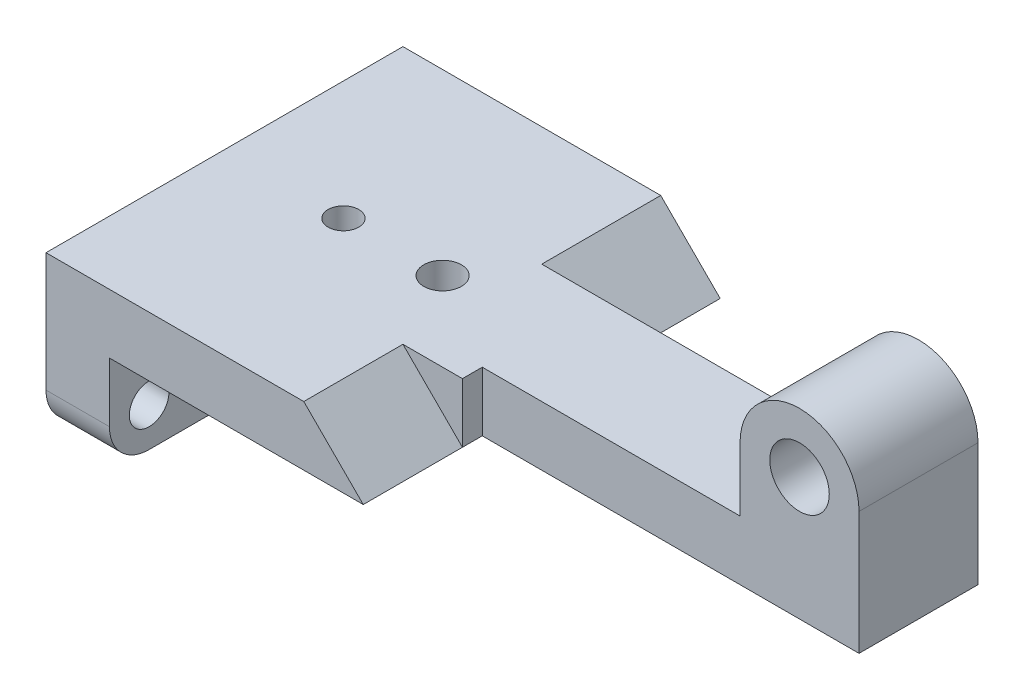
ISO-10303-21;
HEADER;
FILE_DESCRIPTION(('STEP AP214'),'2;1');
FILE_NAME('part.step','',(''),(''),'','','');
FILE_SCHEMA(('AUTOMOTIVE_DESIGN { 1 0 10303 214 1 1 1 1 }'));
ENDSEC;
DATA;
#1=APPLICATION_CONTEXT('core data for automotive mechanical design processes');
#2=APPLICATION_PROTOCOL_DEFINITION('international standard','automotive_design',2000,#1);
#3=PRODUCT_CONTEXT('',#1,'mechanical');
#4=PRODUCT('Part','Part','',(#3));
#5=PRODUCT_RELATED_PRODUCT_CATEGORY('part','',(#4));
#6=PRODUCT_DEFINITION_FORMATION('','',#4);
#7=PRODUCT_DEFINITION_CONTEXT('part definition',#1,'design');
#8=PRODUCT_DEFINITION('design','',#6,#7);
#9=PRODUCT_DEFINITION_SHAPE('','',#8);
#10=(LENGTH_UNIT() NAMED_UNIT(*) SI_UNIT(.MILLI.,.METRE.));
#11=(NAMED_UNIT(*) PLANE_ANGLE_UNIT() SI_UNIT($,.RADIAN.));
#12=(NAMED_UNIT(*) SI_UNIT($,.STERADIAN.) SOLID_ANGLE_UNIT());
#13=UNCERTAINTY_MEASURE_WITH_UNIT(LENGTH_MEASURE(1.E-05),#10,'distance_accuracy_value','');
#14=(GEOMETRIC_REPRESENTATION_CONTEXT(3) GLOBAL_UNCERTAINTY_ASSIGNED_CONTEXT((#13)) GLOBAL_UNIT_ASSIGNED_CONTEXT((#10,
#11,#12)) REPRESENTATION_CONTEXT('',''));
#15=CARTESIAN_POINT('',(0.,0.,0.));
#16=DIRECTION('',(0.,0.,1.));
#17=DIRECTION('',(1.,0.,0.));
#18=AXIS2_PLACEMENT_3D('',#15,#16,#17);
#19=CARTESIAN_POINT('',(80.,-15.,-15.));
#20=DIRECTION('',(1.,0.,0.));
#21=DIRECTION('',(0.,1.,0.));
#22=AXIS2_PLACEMENT_3D('',#19,#20,#21);
#23=PLANE('',#22);
#24=DIRECTION('',(0.,0.,-1.));
#25=VECTOR('',#24,1.);
#26=CARTESIAN_POINT('',(80.,-15.,-15.));
#27=LINE('',#26,#25);
#28=CARTESIAN_POINT('',(80.,-15.,20.));
#29=VERTEX_POINT('',#28);
#30=CARTESIAN_POINT('',(80.,-15.,15.));
#31=VERTEX_POINT('',#30);
#32=EDGE_CURVE('E206',#29,#31,#27,.T.);
#33=ORIENTED_EDGE('',*,*,#32,.T.);
#34=DIRECTION('',(0.,-1.,0.));
#35=VECTOR('',#34,1.);
#36=CARTESIAN_POINT('',(80.,-15.,15.));
#37=LINE('',#36,#35);
#38=CARTESIAN_POINT('',(80.,0.,15.));
#39=VERTEX_POINT('',#38);
#40=EDGE_CURVE('E188',#39,#31,#37,.T.);
#41=ORIENTED_EDGE('',*,*,#40,.F.);
#42=DIRECTION('',(0.,0.,-1.));
#43=VECTOR('',#42,1.);
#44=CARTESIAN_POINT('',(80.,0.,-15.));
#45=LINE('',#44,#43);
#46=CARTESIAN_POINT('',(80.,0.,20.));
#47=VERTEX_POINT('',#46);
#48=EDGE_CURVE('E214',#47,#39,#45,.T.);
#49=ORIENTED_EDGE('',*,*,#48,.F.);
#50=DIRECTION('',(0.,1.,0.));
#51=VECTOR('',#50,1.);
#52=CARTESIAN_POINT('',(80.,-15.,20.));
#53=LINE('',#52,#51);
#54=EDGE_CURVE('E208',#29,#47,#53,.T.);
#55=ORIENTED_EDGE('',*,*,#54,.F.);
#56=EDGE_LOOP('',(#33,#41,#49,#55));
#57=FACE_BOUND('',#56,.T.);
#58=ADVANCED_FACE('F39',(#57),#23,.T.);
#59=CARTESIAN_POINT('',(80.,-15.,45.));
#60=DIRECTION('',(-0.707106781186543,-0.707106781186552,0.));
#61=DIRECTION('',(0.707106781186552,-0.707106781186543,0.));
#62=AXIS2_PLACEMENT_3D('',#59,#60,#61);
#63=PLANE('',#62);
#64=DIRECTION('',(0.,0.,-1.));
#65=VECTOR('',#64,1.);
#66=CARTESIAN_POINT('',(64.9999999999998,0.,45.));
#67=LINE('',#66,#65);
#68=CARTESIAN_POINT('',(64.9999999999998,0.,-15.));
#69=VERTEX_POINT('',#68);
#70=CARTESIAN_POINT('',(64.9999999999998,0.,-45.));
#71=VERTEX_POINT('',#70);
#72=EDGE_CURVE('E233',#69,#71,#67,.T.);
#73=ORIENTED_EDGE('',*,*,#72,.F.);
#74=DIRECTION('',(0.707106781186552,-0.707106781186543,0.));
#75=VECTOR('',#74,1.);
#76=CARTESIAN_POINT('',(80.,-15.,-15.));
#77=LINE('',#76,#75);
#78=CARTESIAN_POINT('',(80.,-15.,-15.));
#79=VERTEX_POINT('',#78);
#80=EDGE_CURVE('E262',#69,#79,#77,.T.);
#81=ORIENTED_EDGE('',*,*,#80,.T.);
#82=DIRECTION('',(0.,0.,-1.));
#83=VECTOR('',#82,1.);
#84=CARTESIAN_POINT('',(80.,-15.,45.));
#85=LINE('',#84,#83);
#86=CARTESIAN_POINT('',(80.,-15.,-45.));
#87=VERTEX_POINT('',#86);
#88=EDGE_CURVE('E246',#79,#87,#85,.T.);
#89=ORIENTED_EDGE('',*,*,#88,.T.);
#90=DIRECTION('',(-0.707106781186552,0.707106781186543,0.));
#91=VECTOR('',#90,1.);
#92=CARTESIAN_POINT('',(80.,-15.,-45.));
#93=LINE('',#92,#91);
#94=EDGE_CURVE('E222',#87,#71,#93,.T.);
#95=ORIENTED_EDGE('',*,*,#94,.T.);
#96=EDGE_LOOP('',(#73,#81,#89,#95));
#97=FACE_BOUND('',#96,.T.);
#98=ADVANCED_FACE('F329',(#97),#63,.F.);
#99=CARTESIAN_POINT('',(64.9999999999998,0.,45.));
#100=DIRECTION('',(0.,-1.,0.));
#101=DIRECTION('',(1.,0.,0.));
#102=AXIS2_PLACEMENT_3D('',#99,#100,#101);
#103=PLANE('',#102);
#104=CARTESIAN_POINT('',(30.,0.,0.));
#105=DIRECTION('',(0.,-1.,0.));
#106=DIRECTION('',(1.,0.,0.));
#107=AXIS2_PLACEMENT_3D('',#104,#105,#106);
#108=CIRCLE('',#107,3.86271087841769);
#109=CARTESIAN_POINT('',(26.1372891215823,0.,0.));
#110=VERTEX_POINT('',#109);
#111=EDGE_CURVE('E284',#110,#110,#108,.T.);
#112=ORIENTED_EDGE('',*,*,#111,.T.);
#113=EDGE_LOOP('',(#112));
#114=FACE_BOUND('',#113,.T.);
#115=CARTESIAN_POINT('',(55.,0.,0.));
#116=DIRECTION('',(0.,-1.,0.));
#117=DIRECTION('',(1.,0.,0.));
#118=AXIS2_PLACEMENT_3D('',#115,#116,#117);
#119=CIRCLE('',#118,4.7402824052039);
#120=CARTESIAN_POINT('',(50.2597175947961,0.,0.));
#121=VERTEX_POINT('',#120);
#122=EDGE_CURVE('E289',#121,#121,#119,.T.);
#123=ORIENTED_EDGE('',*,*,#122,.T.);
#124=EDGE_LOOP('',(#123));
#125=FACE_BOUND('',#124,.T.);
#126=DIRECTION('',(-1.,0.,0.));
#127=VECTOR('',#126,1.);
#128=CARTESIAN_POINT('',(175.,0.,15.));
#129=LINE('',#128,#127);
#130=CARTESIAN_POINT('',(145.,0.,15.));
#131=VERTEX_POINT('',#130);
#132=EDGE_CURVE('E204',#131,#39,#129,.T.);
#133=ORIENTED_EDGE('',*,*,#132,.F.);
#134=DIRECTION('',(0.,0.,-1.));
#135=VECTOR('',#134,1.);
#136=CARTESIAN_POINT('',(145.,0.,45.));
#137=LINE('',#136,#135);
#138=CARTESIAN_POINT('',(145.,0.,-15.));
#139=VERTEX_POINT('',#138);
#140=EDGE_CURVE('E190',#131,#139,#137,.T.);
#141=ORIENTED_EDGE('',*,*,#140,.T.);
#142=DIRECTION('',(-1.,0.,0.));
#143=VECTOR('',#142,1.);
#144=CARTESIAN_POINT('',(64.9999999999998,0.,-15.));
#145=LINE('',#144,#143);
#146=EDGE_CURVE('E173',#139,#69,#145,.T.);
#147=ORIENTED_EDGE('',*,*,#146,.T.);
#148=ORIENTED_EDGE('',*,*,#72,.T.);
#149=DIRECTION('',(-1.,0.,0.));
#150=VECTOR('',#149,1.);
#151=CARTESIAN_POINT('',(64.9999999999998,0.,-45.));
#152=LINE('',#151,#150);
#153=CARTESIAN_POINT('',(0.,0.,-45.));
#154=VERTEX_POINT('',#153);
#155=EDGE_CURVE('E216',#71,#154,#152,.T.);
#156=ORIENTED_EDGE('',*,*,#155,.T.);
#157=DIRECTION('',(0.,0.,-1.));
#158=VECTOR('',#157,1.);
#159=CARTESIAN_POINT('',(0.,0.,45.));
#160=LINE('',#159,#158);
#161=CARTESIAN_POINT('',(0.,0.,45.));
#162=VERTEX_POINT('',#161);
#163=EDGE_CURVE('E256',#162,#154,#160,.T.);
#164=ORIENTED_EDGE('',*,*,#163,.F.);
#165=DIRECTION('',(-1.,0.,0.));
#166=VECTOR('',#165,1.);
#167=CARTESIAN_POINT('',(64.9999999999998,0.,45.));
#168=LINE('',#167,#166);
#169=CARTESIAN_POINT('',(64.9999999999998,0.,45.));
#170=VERTEX_POINT('',#169);
#171=EDGE_CURVE('E219',#170,#162,#168,.T.);
#172=ORIENTED_EDGE('',*,*,#171,.F.);
#173=CARTESIAN_POINT('',(64.9999999999998,0.,20.));
#174=VERTEX_POINT('',#173);
#175=EDGE_CURVE('E243',#170,#174,#67,.T.);
#176=ORIENTED_EDGE('',*,*,#175,.T.);
#177=DIRECTION('',(1.,0.,0.));
#178=VECTOR('',#177,1.);
#179=CARTESIAN_POINT('',(64.9999999999998,0.,20.));
#180=LINE('',#179,#178);
#181=EDGE_CURVE('E210',#174,#47,#180,.T.);
#182=ORIENTED_EDGE('',*,*,#181,.T.);
#183=ORIENTED_EDGE('',*,*,#48,.T.);
#184=EDGE_LOOP('',(#133,#141,#147,#148,#156,#164,#172,#176,#182,#183));
#185=FACE_BOUND('',#184,.T.);
#186=ADVANCED_FACE('F334',(#114,#125,#185),#103,.F.);
#187=CARTESIAN_POINT('',(0.,0.,45.));
#188=DIRECTION('',(1.,0.,0.));
#189=DIRECTION('',(0.,1.,0.));
#190=AXIS2_PLACEMENT_3D('',#187,#188,#189);
#191=PLANE('',#190);
#192=CARTESIAN_POINT('',(0.,-30.,-35.));
#193=DIRECTION('',(1.,0.,0.));
#194=DIRECTION('',(0.,1.,0.));
#195=AXIS2_PLACEMENT_3D('',#192,#193,#194);
#196=CIRCLE('',#195,5.);
#197=CARTESIAN_POINT('',(0.,-35.,-35.));
#198=VERTEX_POINT('',#197);
#199=EDGE_CURVE('E290',#198,#198,#196,.T.);
#200=ORIENTED_EDGE('',*,*,#199,.T.);
#201=EDGE_LOOP('',(#200));
#202=FACE_BOUND('',#201,.T.);
#203=CARTESIAN_POINT('',(0.,-30.,35.));
#204=DIRECTION('',(1.,0.,0.));
#205=DIRECTION('',(0.,1.,0.));
#206=AXIS2_PLACEMENT_3D('',#203,#204,#205);
#207=CIRCLE('',#206,5.);
#208=CARTESIAN_POINT('',(0.,-35.,35.));
#209=VERTEX_POINT('',#208);
#210=EDGE_CURVE('E281',#209,#209,#207,.T.);
#211=ORIENTED_EDGE('',*,*,#210,.T.);
#212=EDGE_LOOP('',(#211));
#213=FACE_BOUND('',#212,.T.);
#214=DIRECTION('',(0.,-1.,0.));
#215=VECTOR('',#214,1.);
#216=CARTESIAN_POINT('',(0.,0.,-45.));
#217=LINE('',#216,#215);
#218=CARTESIAN_POINT('',(0.,-30.,-45.));
#219=VERTEX_POINT('',#218);
#220=EDGE_CURVE('E234',#154,#219,#217,.T.);
#221=ORIENTED_EDGE('',*,*,#220,.T.);
#222=CARTESIAN_POINT('',(0.,-30.,-35.));
#223=DIRECTION('',(1.,0.,0.));
#224=DIRECTION('',(0.,1.,0.));
#225=AXIS2_PLACEMENT_3D('',#222,#223,#224);
#226=CIRCLE('',#225,10.);
#227=CARTESIAN_POINT('',(0.,-40.,-35.));
#228=VERTEX_POINT('',#227);
#229=EDGE_CURVE('E48',#219,#228,#226,.F.);
#230=ORIENTED_EDGE('',*,*,#229,.T.);
#231=DIRECTION('',(0.,0.,-1.));
#232=VECTOR('',#231,1.);
#233=CARTESIAN_POINT('',(0.,-40.,45.));
#234=LINE('',#233,#232);
#235=CARTESIAN_POINT('',(0.,-40.,35.));
#236=VERTEX_POINT('',#235);
#237=EDGE_CURVE('E257',#236,#228,#234,.T.);
#238=ORIENTED_EDGE('',*,*,#237,.F.);
#239=CARTESIAN_POINT('',(0.,-30.,35.));
#240=DIRECTION('',(1.,0.,0.));
#241=DIRECTION('',(0.,1.,0.));
#242=AXIS2_PLACEMENT_3D('',#239,#240,#241);
#243=CIRCLE('',#242,10.);
#244=CARTESIAN_POINT('',(0.,-30.,45.));
#245=VERTEX_POINT('',#244);
#246=EDGE_CURVE('E57',#236,#245,#243,.F.);
#247=ORIENTED_EDGE('',*,*,#246,.T.);
#248=DIRECTION('',(0.,-1.,0.));
#249=VECTOR('',#248,1.);
#250=CARTESIAN_POINT('',(0.,0.,45.));
#251=LINE('',#250,#249);
#252=EDGE_CURVE('E225',#162,#245,#251,.T.);
#253=ORIENTED_EDGE('',*,*,#252,.F.);
#254=ORIENTED_EDGE('',*,*,#163,.T.);
#255=EDGE_LOOP('',(#221,#230,#238,#247,#253,#254));
#256=FACE_BOUND('',#255,.T.);
#257=ADVANCED_FACE('F359',(#202,#213,#256),#191,.F.);
#258=CARTESIAN_POINT('',(0.,-40.,45.));
#259=DIRECTION('',(0.,1.,0.));
#260=DIRECTION('',(0.,0.,1.));
#261=AXIS2_PLACEMENT_3D('',#258,#259,#260);
#262=PLANE('',#261);
#263=ORIENTED_EDGE('',*,*,#237,.T.);
#264=DIRECTION('',(1.,0.,0.));
#265=VECTOR('',#264,1.);
#266=CARTESIAN_POINT('',(0.,-40.,-35.));
#267=LINE('',#266,#265);
#268=CARTESIAN_POINT('',(16.,-40.,-35.));
#269=VERTEX_POINT('',#268);
#270=EDGE_CURVE('E269',#228,#269,#267,.T.);
#271=ORIENTED_EDGE('',*,*,#270,.T.);
#272=DIRECTION('',(0.,0.,-1.));
#273=VECTOR('',#272,1.);
#274=CARTESIAN_POINT('',(16.,-40.,45.));
#275=LINE('',#274,#273);
#276=CARTESIAN_POINT('',(16.,-40.,35.));
#277=VERTEX_POINT('',#276);
#278=EDGE_CURVE('E254',#277,#269,#275,.T.);
#279=ORIENTED_EDGE('',*,*,#278,.F.);
#280=DIRECTION('',(1.,0.,0.));
#281=VECTOR('',#280,1.);
#282=CARTESIAN_POINT('',(0.,-40.,35.));
#283=LINE('',#282,#281);
#284=EDGE_CURVE('E267',#277,#236,#283,.F.);
#285=ORIENTED_EDGE('',*,*,#284,.T.);
#286=EDGE_LOOP('',(#263,#271,#279,#285));
#287=FACE_BOUND('',#286,.T.);
#288=ADVANCED_FACE('F358',(#287),#262,.F.);
#289=CARTESIAN_POINT('',(16.,-40.,45.));
#290=DIRECTION('',(-1.,0.,0.));
#291=DIRECTION('',(0.,0.,1.));
#292=AXIS2_PLACEMENT_3D('',#289,#290,#291);
#293=PLANE('',#292);
#294=CARTESIAN_POINT('',(16.,-30.,-35.));
#295=DIRECTION('',(-1.,0.,0.));
#296=DIRECTION('',(0.,0.,1.));
#297=AXIS2_PLACEMENT_3D('',#294,#295,#296);
#298=CIRCLE('',#297,5.);
#299=CARTESIAN_POINT('',(16.,-35.,-35.));
#300=VERTEX_POINT('',#299);
#301=EDGE_CURVE('E282',#300,#300,#298,.T.);
#302=ORIENTED_EDGE('',*,*,#301,.T.);
#303=EDGE_LOOP('',(#302));
#304=FACE_BOUND('',#303,.T.);
#305=CARTESIAN_POINT('',(16.,-30.,35.));
#306=DIRECTION('',(-1.,0.,0.));
#307=DIRECTION('',(0.,0.,1.));
#308=AXIS2_PLACEMENT_3D('',#305,#306,#307);
#309=CIRCLE('',#308,5.);
#310=CARTESIAN_POINT('',(16.,-35.,35.));
#311=VERTEX_POINT('',#310);
#312=EDGE_CURVE('E278',#311,#311,#309,.T.);
#313=ORIENTED_EDGE('',*,*,#312,.T.);
#314=EDGE_LOOP('',(#313));
#315=FACE_BOUND('',#314,.T.);
#316=ORIENTED_EDGE('',*,*,#278,.T.);
#317=CARTESIAN_POINT('',(16.,-30.,-35.));
#318=DIRECTION('',(-1.,0.,0.));
#319=DIRECTION('',(0.,0.,1.));
#320=AXIS2_PLACEMENT_3D('',#317,#318,#319);
#321=CIRCLE('',#320,10.);
#322=CARTESIAN_POINT('',(16.,-30.,-45.));
#323=VERTEX_POINT('',#322);
#324=EDGE_CURVE('E273',#269,#323,#321,.F.);
#325=ORIENTED_EDGE('',*,*,#324,.T.);
#326=DIRECTION('',(0.,1.,0.));
#327=VECTOR('',#326,1.);
#328=CARTESIAN_POINT('',(16.,-40.,-45.));
#329=LINE('',#328,#327);
#330=CARTESIAN_POINT('',(16.,-15.,-45.));
#331=VERTEX_POINT('',#330);
#332=EDGE_CURVE('E236',#323,#331,#329,.T.);
#333=ORIENTED_EDGE('',*,*,#332,.T.);
#334=DIRECTION('',(0.,0.,-1.));
#335=VECTOR('',#334,1.);
#336=CARTESIAN_POINT('',(16.,-15.,45.));
#337=LINE('',#336,#335);
#338=CARTESIAN_POINT('',(16.,-15.,45.));
#339=VERTEX_POINT('',#338);
#340=EDGE_CURVE('E249',#339,#331,#337,.T.);
#341=ORIENTED_EDGE('',*,*,#340,.F.);
#342=DIRECTION('',(0.,1.,0.));
#343=VECTOR('',#342,1.);
#344=CARTESIAN_POINT('',(16.,-40.,45.));
#345=LINE('',#344,#343);
#346=CARTESIAN_POINT('',(16.,-30.,45.));
#347=VERTEX_POINT('',#346);
#348=EDGE_CURVE('E224',#347,#339,#345,.T.);
#349=ORIENTED_EDGE('',*,*,#348,.F.);
#350=CARTESIAN_POINT('',(16.,-30.,35.));
#351=DIRECTION('',(-1.,0.,0.));
#352=DIRECTION('',(0.,0.,1.));
#353=AXIS2_PLACEMENT_3D('',#350,#351,#352);
#354=CIRCLE('',#353,10.);
#355=EDGE_CURVE('E271',#347,#277,#354,.F.);
#356=ORIENTED_EDGE('',*,*,#355,.T.);
#357=EDGE_LOOP('',(#316,#325,#333,#341,#349,#356));
#358=FACE_BOUND('',#357,.T.);
#359=ADVANCED_FACE('F355',(#304,#315,#358),#293,.F.);
#360=CARTESIAN_POINT('',(16.,-15.,45.));
#361=DIRECTION('',(0.,1.,0.));
#362=DIRECTION('',(-1.,0.,0.));
#363=AXIS2_PLACEMENT_3D('',#360,#361,#362);
#364=PLANE('',#363);
#365=CARTESIAN_POINT('',(30.,-15.,0.));
#366=DIRECTION('',(0.,1.,0.));
#367=DIRECTION('',(-1.,0.,0.));
#368=AXIS2_PLACEMENT_3D('',#365,#366,#367);
#369=CIRCLE('',#368,3.86271087841769);
#370=CARTESIAN_POINT('',(26.1372891215823,-15.,0.));
#371=VERTEX_POINT('',#370);
#372=EDGE_CURVE('E43',#371,#371,#369,.T.);
#373=ORIENTED_EDGE('',*,*,#372,.T.);
#374=EDGE_LOOP('',(#373));
#375=FACE_BOUND('',#374,.T.);
#376=CARTESIAN_POINT('',(55.,-15.,0.));
#377=DIRECTION('',(0.,1.,0.));
#378=DIRECTION('',(-1.,0.,0.));
#379=AXIS2_PLACEMENT_3D('',#376,#377,#378);
#380=CIRCLE('',#379,4.7402824052039);
#381=CARTESIAN_POINT('',(50.2597175947961,-15.,0.));
#382=VERTEX_POINT('',#381);
#383=EDGE_CURVE('E287',#382,#382,#380,.T.);
#384=ORIENTED_EDGE('',*,*,#383,.T.);
#385=EDGE_LOOP('',(#384));
#386=FACE_BOUND('',#385,.T.);
#387=ORIENTED_EDGE('',*,*,#88,.F.);
#388=DIRECTION('',(-1.,0.,0.));
#389=VECTOR('',#388,1.);
#390=CARTESIAN_POINT('',(175.,-15.,-15.));
#391=LINE('',#390,#389);
#392=CARTESIAN_POINT('',(175.,-15.,-15.));
#393=VERTEX_POINT('',#392);
#394=EDGE_CURVE('E200',#393,#79,#391,.T.);
#395=ORIENTED_EDGE('',*,*,#394,.F.);
#396=DIRECTION('',(0.,0.,-1.));
#397=VECTOR('',#396,1.);
#398=CARTESIAN_POINT('',(175.,-15.,-15.));
#399=LINE('',#398,#397);
#400=CARTESIAN_POINT('',(175.,-15.,15.));
#401=VERTEX_POINT('',#400);
#402=EDGE_CURVE('E193',#401,#393,#399,.T.);
#403=ORIENTED_EDGE('',*,*,#402,.F.);
#404=DIRECTION('',(-1.,0.,0.));
#405=VECTOR('',#404,1.);
#406=CARTESIAN_POINT('',(175.,-15.,15.));
#407=LINE('',#406,#405);
#408=EDGE_CURVE('E205',#401,#31,#407,.T.);
#409=ORIENTED_EDGE('',*,*,#408,.T.);
#410=ORIENTED_EDGE('',*,*,#32,.F.);
#411=CARTESIAN_POINT('',(80.,-15.,45.));
#412=VERTEX_POINT('',#411);
#413=EDGE_CURVE('E250',#412,#29,#85,.T.);
#414=ORIENTED_EDGE('',*,*,#413,.F.);
#415=DIRECTION('',(1.,0.,0.));
#416=VECTOR('',#415,1.);
#417=CARTESIAN_POINT('',(16.,-15.,45.));
#418=LINE('',#417,#416);
#419=EDGE_CURVE('E227',#339,#412,#418,.T.);
#420=ORIENTED_EDGE('',*,*,#419,.F.);
#421=ORIENTED_EDGE('',*,*,#340,.T.);
#422=DIRECTION('',(1.,0.,0.));
#423=VECTOR('',#422,1.);
#424=CARTESIAN_POINT('',(16.,-15.,-45.));
#425=LINE('',#424,#423);
#426=EDGE_CURVE('E238',#331,#87,#425,.T.);
#427=ORIENTED_EDGE('',*,*,#426,.T.);
#428=EDGE_LOOP('',(#387,#395,#403,#409,#410,#414,#420,#421,#427));
#429=FACE_BOUND('',#428,.T.);
#430=ADVANCED_FACE('F346',(#375,#386,#429),#364,.F.);
#431=ORIENTED_EDGE('',*,*,#413,.T.);
#432=DIRECTION('',(-0.707106781186552,0.707106781186543,0.));
#433=VECTOR('',#432,1.);
#434=CARTESIAN_POINT('',(80.,-15.,20.));
#435=LINE('',#434,#433);
#436=EDGE_CURVE('E265',#29,#174,#435,.T.);
#437=ORIENTED_EDGE('',*,*,#436,.T.);
#438=ORIENTED_EDGE('',*,*,#175,.F.);
#439=DIRECTION('',(-0.707106781186552,0.707106781186543,0.));
#440=VECTOR('',#439,1.);
#441=CARTESIAN_POINT('',(80.,-15.,45.));
#442=LINE('',#441,#440);
#443=EDGE_CURVE('E230',#412,#170,#442,.T.);
#444=ORIENTED_EDGE('',*,*,#443,.F.);
#445=EDGE_LOOP('',(#431,#437,#438,#444));
#446=FACE_BOUND('',#445,.T.);
#447=ADVANCED_FACE('F336',(#446),#63,.F.);
#448=CARTESIAN_POINT('',(0.,0.,45.));
#449=DIRECTION('',(0.,0.,1.));
#450=DIRECTION('',(1.,0.,0.));
#451=AXIS2_PLACEMENT_3D('',#448,#449,#450);
#452=PLANE('',#451);
#453=ORIENTED_EDGE('',*,*,#252,.T.);
#454=DIRECTION('',(1.,0.,0.));
#455=VECTOR('',#454,1.);
#456=CARTESIAN_POINT('',(16.,-30.,45.));
#457=LINE('',#456,#455);
#458=EDGE_CURVE('E11',#245,#347,#457,.T.);
#459=ORIENTED_EDGE('',*,*,#458,.T.);
#460=ORIENTED_EDGE('',*,*,#348,.T.);
#461=ORIENTED_EDGE('',*,*,#419,.T.);
#462=ORIENTED_EDGE('',*,*,#443,.T.);
#463=ORIENTED_EDGE('',*,*,#171,.T.);
#464=EDGE_LOOP('',(#453,#459,#460,#461,#462,#463));
#465=FACE_BOUND('',#464,.T.);
#466=ADVANCED_FACE('F338',(#465),#452,.T.);
#467=CARTESIAN_POINT('',(0.,0.,-45.));
#468=DIRECTION('',(0.,0.,1.));
#469=DIRECTION('',(1.,0.,0.));
#470=AXIS2_PLACEMENT_3D('',#467,#468,#469);
#471=PLANE('',#470);
#472=ORIENTED_EDGE('',*,*,#332,.F.);
#473=DIRECTION('',(1.,0.,0.));
#474=VECTOR('',#473,1.);
#475=CARTESIAN_POINT('',(0.,-30.,-45.));
#476=LINE('',#475,#474);
#477=EDGE_CURVE('E61',#323,#219,#476,.F.);
#478=ORIENTED_EDGE('',*,*,#477,.T.);
#479=ORIENTED_EDGE('',*,*,#220,.F.);
#480=ORIENTED_EDGE('',*,*,#155,.F.);
#481=ORIENTED_EDGE('',*,*,#94,.F.);
#482=ORIENTED_EDGE('',*,*,#426,.F.);
#483=EDGE_LOOP('',(#472,#478,#479,#480,#481,#482));
#484=FACE_BOUND('',#483,.T.);
#485=ADVANCED_FACE('F344',(#484),#471,.F.);
#486=CARTESIAN_POINT('',(64.9999999999998,-15.,-15.));
#487=DIRECTION('',(0.,0.,-1.));
#488=DIRECTION('',(-1.,0.,0.));
#489=AXIS2_PLACEMENT_3D('',#486,#487,#488);
#490=PLANE('',#489);
#491=CARTESIAN_POINT('',(160.,16.,-15.));
#492=DIRECTION('',(0.,0.,1.));
#493=DIRECTION('',(1.,0.,0.));
#494=AXIS2_PLACEMENT_3D('',#491,#492,#493);
#495=CIRCLE('',#494,15.);
#496=CARTESIAN_POINT('',(175.,16.,-15.));
#497=VERTEX_POINT('',#496);
#498=CARTESIAN_POINT('',(145.,16.,-15.));
#499=VERTEX_POINT('',#498);
#500=EDGE_CURVE('E171',#497,#499,#495,.T.);
#501=ORIENTED_EDGE('',*,*,#500,.F.);
#502=DIRECTION('',(0.,1.,0.));
#503=VECTOR('',#502,1.);
#504=CARTESIAN_POINT('',(175.,-15.,-15.));
#505=LINE('',#504,#503);
#506=EDGE_CURVE('E192',#393,#497,#505,.T.);
#507=ORIENTED_EDGE('',*,*,#506,.F.);
#508=ORIENTED_EDGE('',*,*,#394,.T.);
#509=ORIENTED_EDGE('',*,*,#80,.F.);
#510=ORIENTED_EDGE('',*,*,#146,.F.);
#511=DIRECTION('',(0.,-1.,0.));
#512=VECTOR('',#511,1.);
#513=CARTESIAN_POINT('',(145.,16.,-15.));
#514=LINE('',#513,#512);
#515=EDGE_CURVE('E156',#499,#139,#514,.T.);
#516=ORIENTED_EDGE('',*,*,#515,.F.);
#517=EDGE_LOOP('',(#501,#507,#508,#509,#510,#516));
#518=FACE_BOUND('',#517,.T.);
#519=CARTESIAN_POINT('',(160.,16.,-15.));
#520=DIRECTION('',(0.,0.,1.));
#521=DIRECTION('',(1.,0.,0.));
#522=AXIS2_PLACEMENT_3D('',#519,#520,#521);
#523=CIRCLE('',#522,7.50000000000001);
#524=CARTESIAN_POINT('',(167.5,16.,-15.));
#525=VERTEX_POINT('',#524);
#526=EDGE_CURVE('E184',#525,#525,#523,.T.);
#527=ORIENTED_EDGE('',*,*,#526,.T.);
#528=EDGE_LOOP('',(#527));
#529=FACE_BOUND('',#528,.T.);
#530=ADVANCED_FACE('F166',(#518,#529),#490,.T.);
#531=CARTESIAN_POINT('',(64.9999999999998,-15.,20.));
#532=DIRECTION('',(0.,0.,1.));
#533=DIRECTION('',(1.,0.,0.));
#534=AXIS2_PLACEMENT_3D('',#531,#532,#533);
#535=PLANE('',#534);
#536=ORIENTED_EDGE('',*,*,#436,.F.);
#537=ORIENTED_EDGE('',*,*,#54,.T.);
#538=ORIENTED_EDGE('',*,*,#181,.F.);
#539=EDGE_LOOP('',(#536,#537,#538));
#540=FACE_BOUND('',#539,.T.);
#541=ADVANCED_FACE('F313',(#540),#535,.T.);
#542=CARTESIAN_POINT('',(175.,-15.,15.));
#543=DIRECTION('',(0.,0.,-1.));
#544=DIRECTION('',(0.,1.,0.));
#545=AXIS2_PLACEMENT_3D('',#542,#543,#544);
#546=PLANE('',#545);
#547=ORIENTED_EDGE('',*,*,#408,.F.);
#548=DIRECTION('',(0.,-1.,0.));
#549=VECTOR('',#548,1.);
#550=CARTESIAN_POINT('',(175.,-15.,15.));
#551=LINE('',#550,#549);
#552=CARTESIAN_POINT('',(175.,16.,15.));
#553=VERTEX_POINT('',#552);
#554=EDGE_CURVE('E194',#553,#401,#551,.T.);
#555=ORIENTED_EDGE('',*,*,#554,.F.);
#556=CARTESIAN_POINT('',(160.,16.,15.));
#557=DIRECTION('',(0.,0.,1.));
#558=DIRECTION('',(1.,0.,0.));
#559=AXIS2_PLACEMENT_3D('',#556,#557,#558);
#560=CIRCLE('',#559,15.);
#561=CARTESIAN_POINT('',(145.,16.,15.));
#562=VERTEX_POINT('',#561);
#563=EDGE_CURVE('E177',#553,#562,#560,.T.);
#564=ORIENTED_EDGE('',*,*,#563,.T.);
#565=DIRECTION('',(0.,-1.,0.));
#566=VECTOR('',#565,1.);
#567=CARTESIAN_POINT('',(145.,16.,15.));
#568=LINE('',#567,#566);
#569=EDGE_CURVE('E157',#562,#131,#568,.T.);
#570=ORIENTED_EDGE('',*,*,#569,.T.);
#571=ORIENTED_EDGE('',*,*,#132,.T.);
#572=ORIENTED_EDGE('',*,*,#40,.T.);
#573=EDGE_LOOP('',(#547,#555,#564,#570,#571,#572));
#574=FACE_BOUND('',#573,.T.);
#575=CARTESIAN_POINT('',(160.,16.,15.));
#576=DIRECTION('',(0.,0.,1.));
#577=DIRECTION('',(1.,0.,0.));
#578=AXIS2_PLACEMENT_3D('',#575,#576,#577);
#579=CIRCLE('',#578,7.50000000000001);
#580=CARTESIAN_POINT('',(167.5,16.,15.));
#581=VERTEX_POINT('',#580);
#582=EDGE_CURVE('E185',#581,#581,#579,.T.);
#583=ORIENTED_EDGE('',*,*,#582,.F.);
#584=EDGE_LOOP('',(#583));
#585=FACE_BOUND('',#584,.T.);
#586=ADVANCED_FACE('F311',(#574,#585),#546,.F.);
#587=CARTESIAN_POINT('',(175.,0.,0.));
#588=DIRECTION('',(1.,0.,0.));
#589=DIRECTION('',(0.,0.,-1.));
#590=AXIS2_PLACEMENT_3D('',#587,#588,#589);
#591=PLANE('',#590);
#592=ORIENTED_EDGE('',*,*,#506,.T.);
#593=DIRECTION('',(0.,0.,1.));
#594=VECTOR('',#593,1.);
#595=CARTESIAN_POINT('',(175.,16.,-15.));
#596=LINE('',#595,#594);
#597=EDGE_CURVE('E161',#497,#553,#596,.T.);
#598=ORIENTED_EDGE('',*,*,#597,.T.);
#599=ORIENTED_EDGE('',*,*,#554,.T.);
#600=ORIENTED_EDGE('',*,*,#402,.T.);
#601=EDGE_LOOP('',(#592,#598,#599,#600));
#602=FACE_BOUND('',#601,.T.);
#603=ADVANCED_FACE('F312',(#602),#591,.T.);
#604=CARTESIAN_POINT('',(145.,16.,-15.));
#605=DIRECTION('',(-1.,0.,0.));
#606=DIRECTION('',(0.,0.,1.));
#607=AXIS2_PLACEMENT_3D('',#604,#605,#606);
#608=PLANE('',#607);
#609=ORIENTED_EDGE('',*,*,#140,.F.);
#610=ORIENTED_EDGE('',*,*,#569,.F.);
#611=DIRECTION('',(0.,0.,1.));
#612=VECTOR('',#611,1.);
#613=CARTESIAN_POINT('',(145.,16.,-15.));
#614=LINE('',#613,#612);
#615=EDGE_CURVE('E155',#499,#562,#614,.T.);
#616=ORIENTED_EDGE('',*,*,#615,.F.);
#617=ORIENTED_EDGE('',*,*,#515,.T.);
#618=EDGE_LOOP('',(#609,#610,#616,#617));
#619=FACE_BOUND('',#618,.T.);
#620=ADVANCED_FACE('F152',(#619),#608,.T.);
#621=CARTESIAN_POINT('',(160.,16.,-15.));
#622=DIRECTION('',(0.,0.,1.));
#623=DIRECTION('',(1.,0.,0.));
#624=AXIS2_PLACEMENT_3D('',#621,#622,#623);
#625=CYLINDRICAL_SURFACE('',#624,15.);
#626=ORIENTED_EDGE('',*,*,#563,.F.);
#627=ORIENTED_EDGE('',*,*,#597,.F.);
#628=ORIENTED_EDGE('',*,*,#500,.T.);
#629=ORIENTED_EDGE('',*,*,#615,.T.);
#630=EDGE_LOOP('',(#626,#627,#628,#629));
#631=FACE_BOUND('',#630,.T.);
#632=ADVANCED_FACE('F176',(#631),#625,.T.);
#633=CARTESIAN_POINT('',(160.,16.,-15.));
#634=DIRECTION('',(0.,0.,1.));
#635=DIRECTION('',(1.,0.,0.));
#636=AXIS2_PLACEMENT_3D('',#633,#634,#635);
#637=CYLINDRICAL_SURFACE('',#636,7.50000000000001);
#638=ORIENTED_EDGE('',*,*,#526,.F.);
#639=EDGE_LOOP('',(#638));
#640=FACE_BOUND('',#639,.T.);
#641=ORIENTED_EDGE('',*,*,#582,.T.);
#642=EDGE_LOOP('',(#641));
#643=FACE_BOUND('',#642,.T.);
#644=ADVANCED_FACE('F307',(#640,#643),#637,.F.);
#645=CARTESIAN_POINT('',(0.,-30.,-35.));
#646=DIRECTION('',(1.,0.,0.));
#647=DIRECTION('',(0.,0.,-1.));
#648=AXIS2_PLACEMENT_3D('',#645,#646,#647);
#649=CYLINDRICAL_SURFACE('',#648,10.);
#650=ORIENTED_EDGE('',*,*,#229,.F.);
#651=ORIENTED_EDGE('',*,*,#477,.F.);
#652=ORIENTED_EDGE('',*,*,#324,.F.);
#653=ORIENTED_EDGE('',*,*,#270,.F.);
#654=EDGE_LOOP('',(#650,#651,#652,#653));
#655=FACE_BOUND('',#654,.T.);
#656=ADVANCED_FACE('F370',(#655),#649,.T.);
#657=CARTESIAN_POINT('',(0.,-30.,35.));
#658=DIRECTION('',(-1.,0.,0.));
#659=DIRECTION('',(0.,0.,1.));
#660=AXIS2_PLACEMENT_3D('',#657,#658,#659);
#661=CYLINDRICAL_SURFACE('',#660,10.);
#662=ORIENTED_EDGE('',*,*,#246,.F.);
#663=ORIENTED_EDGE('',*,*,#284,.F.);
#664=ORIENTED_EDGE('',*,*,#355,.F.);
#665=ORIENTED_EDGE('',*,*,#458,.F.);
#666=EDGE_LOOP('',(#662,#663,#664,#665));
#667=FACE_BOUND('',#666,.T.);
#668=ADVANCED_FACE('F41',(#667),#661,.T.);
#669=CARTESIAN_POINT('',(60.,-30.,35.));
#670=DIRECTION('',(-1.,0.,0.));
#671=DIRECTION('',(0.,-1.,0.));
#672=AXIS2_PLACEMENT_3D('',#669,#670,#671);
#673=CYLINDRICAL_SURFACE('',#672,5.);
#674=CARTESIAN_POINT('',(16.,-35.,35.));
#675=CARTESIAN_POINT('',(15.8333333333333,-35.,35.));
#676=CARTESIAN_POINT('',(15.6666666666667,-35.,35.));
#677=CARTESIAN_POINT('',(15.3333333333333,-35.,35.));
#678=CARTESIAN_POINT('',(15.1666666666667,-35.,35.));
#679=CARTESIAN_POINT('',(14.8333333333333,-35.,35.));
#680=CARTESIAN_POINT('',(14.6666666666667,-35.,35.));
#681=CARTESIAN_POINT('',(14.3333333333333,-35.,35.));
#682=CARTESIAN_POINT('',(14.1666666666667,-35.,35.));
#683=CARTESIAN_POINT('',(13.8333333333333,-35.,35.));
#684=CARTESIAN_POINT('',(13.6666666666667,-35.,35.));
#685=CARTESIAN_POINT('',(13.3333333333333,-35.,35.));
#686=CARTESIAN_POINT('',(13.1666666666667,-35.,35.));
#687=CARTESIAN_POINT('',(12.8333333333333,-35.,35.));
#688=CARTESIAN_POINT('',(12.6666666666667,-35.,35.));
#689=CARTESIAN_POINT('',(12.3333333333333,-35.,35.));
#690=CARTESIAN_POINT('',(12.1666666666667,-35.,35.));
#691=CARTESIAN_POINT('',(11.8333333333333,-35.,35.));
#692=CARTESIAN_POINT('',(11.6666666666667,-35.,35.));
#693=CARTESIAN_POINT('',(11.3333333333333,-35.,35.));
#694=CARTESIAN_POINT('',(11.1666666666667,-35.,35.));
#695=CARTESIAN_POINT('',(10.8333333333333,-35.,35.));
#696=CARTESIAN_POINT('',(10.6666666666667,-35.,35.));
#697=CARTESIAN_POINT('',(10.3333333333333,-35.,35.));
#698=CARTESIAN_POINT('',(10.1666666666667,-35.,35.));
#699=CARTESIAN_POINT('',(9.83333333333334,-35.,35.));
#700=CARTESIAN_POINT('',(9.66666666666667,-35.,35.));
#701=CARTESIAN_POINT('',(9.33333333333334,-35.,35.));
#702=CARTESIAN_POINT('',(9.16666666666667,-35.,35.));
#703=CARTESIAN_POINT('',(8.83333333333334,-35.,35.));
#704=CARTESIAN_POINT('',(8.66666666666667,-35.,35.));
#705=CARTESIAN_POINT('',(8.33333333333334,-35.,35.));
#706=CARTESIAN_POINT('',(8.16666666666667,-35.,35.));
#707=CARTESIAN_POINT('',(7.83333333333334,-35.,35.));
#708=CARTESIAN_POINT('',(7.66666666666667,-35.,35.));
#709=CARTESIAN_POINT('',(7.33333333333334,-35.,35.));
#710=CARTESIAN_POINT('',(7.16666666666667,-35.,35.));
#711=CARTESIAN_POINT('',(6.83333333333334,-35.,35.));
#712=CARTESIAN_POINT('',(6.66666666666667,-35.,35.));
#713=CARTESIAN_POINT('',(6.33333333333334,-35.,35.));
#714=CARTESIAN_POINT('',(6.16666666666667,-35.,35.));
#715=CARTESIAN_POINT('',(5.83333333333334,-35.,35.));
#716=CARTESIAN_POINT('',(5.66666666666667,-35.,35.));
#717=CARTESIAN_POINT('',(5.33333333333334,-35.,35.));
#718=CARTESIAN_POINT('',(5.16666666666668,-35.,35.));
#719=CARTESIAN_POINT('',(4.83333333333334,-35.,35.));
#720=CARTESIAN_POINT('',(4.66666666666668,-35.,35.));
#721=CARTESIAN_POINT('',(4.33333333333334,-35.,35.));
#722=CARTESIAN_POINT('',(4.16666666666668,-35.,35.));
#723=CARTESIAN_POINT('',(3.83333333333334,-35.,35.));
#724=CARTESIAN_POINT('',(3.66666666666668,-35.,35.));
#725=CARTESIAN_POINT('',(3.33333333333334,-35.,35.));
#726=CARTESIAN_POINT('',(3.16666666666668,-35.,35.));
#727=CARTESIAN_POINT('',(2.83333333333334,-35.,35.));
#728=CARTESIAN_POINT('',(2.66666666666668,-35.,35.));
#729=CARTESIAN_POINT('',(2.33333333333334,-35.,35.));
#730=CARTESIAN_POINT('',(2.16666666666668,-35.,35.));
#731=CARTESIAN_POINT('',(1.83333333333334,-35.,35.));
#732=CARTESIAN_POINT('',(1.66666666666667,-35.,35.));
#733=CARTESIAN_POINT('',(1.33333333333334,-35.,35.));
#734=CARTESIAN_POINT('',(1.16666666666667,-35.,35.));
#735=CARTESIAN_POINT('',(0.833333333333341,-35.,35.));
#736=CARTESIAN_POINT('',(0.666666666666674,-35.,35.));
#737=CARTESIAN_POINT('',(0.333333333333341,-35.,35.));
#738=CARTESIAN_POINT('',(0.166666666666674,-35.,35.));
#739=CARTESIAN_POINT('',(0.,-35.,35.));
#740=B_SPLINE_CURVE_WITH_KNOTS('',3,(#674,#675,#676,#677,#678,#679,#680,#681,#682,#683,#684,
#685,#686,#687,#688,#689,#690,#691,#692,#693,#694,#695,#696,#697,#698,#699,#700,#701,#702,#703,
#704,#705,#706,#707,#708,#709,#710,#711,#712,#713,#714,#715,#716,#717,#718,#719,#720,#721,#722,
#723,#724,#725,#726,#727,#728,#729,#730,#731,#732,#733,#734,#735,#736,#737,#738,#739),
.UNSPECIFIED.,.F.,.F.,(4,2,2,2,2,2,2,2,2,2,2,2,2,2,2,2,2,2,2,2,2,2,2,2,2,2,2,2,2,2,2,2,4),(0.,
0.5,1.,1.5,2.,2.5,3.,3.5,4.,4.5,5.,5.5,6.,6.5,7.,7.5,8.,8.5,9.,9.5,10.,10.5,11.,11.5,12.,12.5,
13.,13.5,14.,14.5,15.,15.5,16.),.UNSPECIFIED.);
#741=EDGE_CURVE('BSEAM373',#311,#209,#740,.T.);
#742=ORIENTED_EDGE('',*,*,#312,.F.);
#743=ORIENTED_EDGE('',*,*,#210,.F.);
#744=ORIENTED_EDGE('',*,*,#741,.T.);
#745=ORIENTED_EDGE('',*,*,#741,.F.);
#746=EDGE_LOOP('',(#742,#744,#743,#745));
#747=FACE_BOUND('',#746,.T.);
#748=ADVANCED_FACE('F373',(#747),#673,.F.);
#749=CARTESIAN_POINT('',(60.,-30.,-35.));
#750=DIRECTION('',(-1.,0.,0.));
#751=DIRECTION('',(0.,-1.,0.));
#752=AXIS2_PLACEMENT_3D('',#749,#750,#751);
#753=CYLINDRICAL_SURFACE('',#752,5.);
#754=CARTESIAN_POINT('',(16.,-35.,-35.));
#755=CARTESIAN_POINT('',(15.8333333333333,-35.,-35.));
#756=CARTESIAN_POINT('',(15.6666666666667,-35.,-35.));
#757=CARTESIAN_POINT('',(15.3333333333333,-35.,-35.));
#758=CARTESIAN_POINT('',(15.1666666666667,-35.,-35.));
#759=CARTESIAN_POINT('',(14.8333333333333,-35.,-35.));
#760=CARTESIAN_POINT('',(14.6666666666667,-35.,-35.));
#761=CARTESIAN_POINT('',(14.3333333333333,-35.,-35.));
#762=CARTESIAN_POINT('',(14.1666666666667,-35.,-35.));
#763=CARTESIAN_POINT('',(13.8333333333333,-35.,-35.));
#764=CARTESIAN_POINT('',(13.6666666666667,-35.,-35.));
#765=CARTESIAN_POINT('',(13.3333333333333,-35.,-35.));
#766=CARTESIAN_POINT('',(13.1666666666667,-35.,-35.));
#767=CARTESIAN_POINT('',(12.8333333333333,-35.,-35.));
#768=CARTESIAN_POINT('',(12.6666666666667,-35.,-35.));
#769=CARTESIAN_POINT('',(12.3333333333333,-35.,-35.));
#770=CARTESIAN_POINT('',(12.1666666666667,-35.,-35.));
#771=CARTESIAN_POINT('',(11.8333333333333,-35.,-35.));
#772=CARTESIAN_POINT('',(11.6666666666667,-35.,-35.));
#773=CARTESIAN_POINT('',(11.3333333333333,-35.,-35.));
#774=CARTESIAN_POINT('',(11.1666666666667,-35.,-35.));
#775=CARTESIAN_POINT('',(10.8333333333333,-35.,-35.));
#776=CARTESIAN_POINT('',(10.6666666666667,-35.,-35.));
#777=CARTESIAN_POINT('',(10.3333333333333,-35.,-35.));
#778=CARTESIAN_POINT('',(10.1666666666667,-35.,-35.));
#779=CARTESIAN_POINT('',(9.83333333333334,-35.,-35.));
#780=CARTESIAN_POINT('',(9.66666666666667,-35.,-35.));
#781=CARTESIAN_POINT('',(9.33333333333334,-35.,-35.));
#782=CARTESIAN_POINT('',(9.16666666666667,-35.,-35.));
#783=CARTESIAN_POINT('',(8.83333333333334,-35.,-35.));
#784=CARTESIAN_POINT('',(8.66666666666667,-35.,-35.));
#785=CARTESIAN_POINT('',(8.33333333333334,-35.,-35.));
#786=CARTESIAN_POINT('',(8.16666666666667,-35.,-35.));
#787=CARTESIAN_POINT('',(7.83333333333334,-35.,-35.));
#788=CARTESIAN_POINT('',(7.66666666666667,-35.,-35.));
#789=CARTESIAN_POINT('',(7.33333333333334,-35.,-35.));
#790=CARTESIAN_POINT('',(7.16666666666667,-35.,-35.));
#791=CARTESIAN_POINT('',(6.83333333333334,-35.,-35.));
#792=CARTESIAN_POINT('',(6.66666666666667,-35.,-35.));
#793=CARTESIAN_POINT('',(6.33333333333334,-35.,-35.));
#794=CARTESIAN_POINT('',(6.16666666666667,-35.,-35.));
#795=CARTESIAN_POINT('',(5.83333333333334,-35.,-35.));
#796=CARTESIAN_POINT('',(5.66666666666667,-35.,-35.));
#797=CARTESIAN_POINT('',(5.33333333333334,-35.,-35.));
#798=CARTESIAN_POINT('',(5.16666666666668,-35.,-35.));
#799=CARTESIAN_POINT('',(4.83333333333334,-35.,-35.));
#800=CARTESIAN_POINT('',(4.66666666666668,-35.,-35.));
#801=CARTESIAN_POINT('',(4.33333333333334,-35.,-35.));
#802=CARTESIAN_POINT('',(4.16666666666668,-35.,-35.));
#803=CARTESIAN_POINT('',(3.83333333333334,-35.,-35.));
#804=CARTESIAN_POINT('',(3.66666666666668,-35.,-35.));
#805=CARTESIAN_POINT('',(3.33333333333334,-35.,-35.));
#806=CARTESIAN_POINT('',(3.16666666666668,-35.,-35.));
#807=CARTESIAN_POINT('',(2.83333333333334,-35.,-35.));
#808=CARTESIAN_POINT('',(2.66666666666668,-35.,-35.));
#809=CARTESIAN_POINT('',(2.33333333333334,-35.,-35.));
#810=CARTESIAN_POINT('',(2.16666666666668,-35.,-35.));
#811=CARTESIAN_POINT('',(1.83333333333334,-35.,-35.));
#812=CARTESIAN_POINT('',(1.66666666666667,-35.,-35.));
#813=CARTESIAN_POINT('',(1.33333333333334,-35.,-35.));
#814=CARTESIAN_POINT('',(1.16666666666667,-35.,-35.));
#815=CARTESIAN_POINT('',(0.833333333333341,-35.,-35.));
#816=CARTESIAN_POINT('',(0.666666666666674,-35.,-35.));
#817=CARTESIAN_POINT('',(0.333333333333341,-35.,-35.));
#818=CARTESIAN_POINT('',(0.166666666666674,-35.,-35.));
#819=CARTESIAN_POINT('',(0.,-35.,-35.));
#820=B_SPLINE_CURVE_WITH_KNOTS('',3,(#754,#755,#756,#757,#758,#759,#760,#761,#762,#763,#764,
#765,#766,#767,#768,#769,#770,#771,#772,#773,#774,#775,#776,#777,#778,#779,#780,#781,#782,#783,
#784,#785,#786,#787,#788,#789,#790,#791,#792,#793,#794,#795,#796,#797,#798,#799,#800,#801,#802,
#803,#804,#805,#806,#807,#808,#809,#810,#811,#812,#813,#814,#815,#816,#817,#818,#819),
.UNSPECIFIED.,.F.,.F.,(4,2,2,2,2,2,2,2,2,2,2,2,2,2,2,2,2,2,2,2,2,2,2,2,2,2,2,2,2,2,2,2,4),(0.,
0.5,1.,1.5,2.,2.5,3.,3.5,4.,4.5,5.,5.5,6.,6.5,7.,7.5,8.,8.5,9.,9.5,10.,10.5,11.,11.5,12.,12.5,
13.,13.5,14.,14.5,15.,15.5,16.),.UNSPECIFIED.);
#821=EDGE_CURVE('BSEAM447',#300,#198,#820,.T.);
#822=ORIENTED_EDGE('',*,*,#301,.F.);
#823=ORIENTED_EDGE('',*,*,#199,.F.);
#824=ORIENTED_EDGE('',*,*,#821,.T.);
#825=ORIENTED_EDGE('',*,*,#821,.F.);
#826=EDGE_LOOP('',(#822,#824,#823,#825));
#827=FACE_BOUND('',#826,.T.);
#828=ADVANCED_FACE('F447',(#827),#753,.F.);
#829=CARTESIAN_POINT('',(55.,-60.,0.));
#830=DIRECTION('',(0.,1.,0.));
#831=DIRECTION('',(-1.,0.,0.));
#832=AXIS2_PLACEMENT_3D('',#829,#830,#831);
#833=CYLINDRICAL_SURFACE('',#832,4.7402824052039);
#834=CARTESIAN_POINT('',(50.2597175947961,-15.,0.));
#835=CARTESIAN_POINT('',(50.2597175947961,-14.84375,0.));
#836=CARTESIAN_POINT('',(50.2597175947961,-14.6875,0.));
#837=CARTESIAN_POINT('',(50.2597175947961,-14.375,0.));
#838=CARTESIAN_POINT('',(50.2597175947961,-14.21875,0.));
#839=CARTESIAN_POINT('',(50.2597175947961,-13.90625,0.));
#840=CARTESIAN_POINT('',(50.2597175947961,-13.75,0.));
#841=CARTESIAN_POINT('',(50.2597175947961,-13.4375,0.));
#842=CARTESIAN_POINT('',(50.2597175947961,-13.28125,0.));
#843=CARTESIAN_POINT('',(50.2597175947961,-12.96875,0.));
#844=CARTESIAN_POINT('',(50.2597175947961,-12.8125,0.));
#845=CARTESIAN_POINT('',(50.2597175947961,-12.5,0.));
#846=CARTESIAN_POINT('',(50.2597175947961,-12.34375,0.));
#847=CARTESIAN_POINT('',(50.2597175947961,-12.03125,0.));
#848=CARTESIAN_POINT('',(50.2597175947961,-11.875,0.));
#849=CARTESIAN_POINT('',(50.2597175947961,-11.5625,0.));
#850=CARTESIAN_POINT('',(50.2597175947961,-11.40625,0.));
#851=CARTESIAN_POINT('',(50.2597175947961,-11.09375,0.));
#852=CARTESIAN_POINT('',(50.2597175947961,-10.9375,0.));
#853=CARTESIAN_POINT('',(50.2597175947961,-10.625,0.));
#854=CARTESIAN_POINT('',(50.2597175947961,-10.46875,0.));
#855=CARTESIAN_POINT('',(50.2597175947961,-10.15625,0.));
#856=CARTESIAN_POINT('',(50.2597175947961,-10.,0.));
#857=CARTESIAN_POINT('',(50.2597175947961,-9.68750000000001,0.));
#858=CARTESIAN_POINT('',(50.2597175947961,-9.53125000000001,0.));
#859=CARTESIAN_POINT('',(50.2597175947961,-9.21875000000001,0.));
#860=CARTESIAN_POINT('',(50.2597175947961,-9.06250000000001,0.));
#861=CARTESIAN_POINT('',(50.2597175947961,-8.75000000000001,0.));
#862=CARTESIAN_POINT('',(50.2597175947961,-8.59375000000001,0.));
#863=CARTESIAN_POINT('',(50.2597175947961,-8.28125000000001,0.));
#864=CARTESIAN_POINT('',(50.2597175947961,-8.12500000000001,0.));
#865=CARTESIAN_POINT('',(50.2597175947961,-7.81250000000001,0.));
#866=CARTESIAN_POINT('',(50.2597175947961,-7.65625000000001,0.));
#867=CARTESIAN_POINT('',(50.2597175947961,-7.34375000000001,0.));
#868=CARTESIAN_POINT('',(50.2597175947961,-7.1875,0.));
#869=CARTESIAN_POINT('',(50.2597175947961,-6.875,0.));
#870=CARTESIAN_POINT('',(50.2597175947961,-6.71875000000001,0.));
#871=CARTESIAN_POINT('',(50.2597175947961,-6.40625000000001,0.));
#872=CARTESIAN_POINT('',(50.2597175947961,-6.25000000000001,0.));
#873=CARTESIAN_POINT('',(50.2597175947961,-5.93750000000001,0.));
#874=CARTESIAN_POINT('',(50.2597175947961,-5.78125000000001,0.));
#875=CARTESIAN_POINT('',(50.2597175947961,-5.46875,0.));
#876=CARTESIAN_POINT('',(50.2597175947961,-5.3125,0.));
#877=CARTESIAN_POINT('',(50.2597175947961,-5.,0.));
#878=CARTESIAN_POINT('',(50.2597175947961,-4.84375,0.));
#879=CARTESIAN_POINT('',(50.2597175947961,-4.53125000000001,0.));
#880=CARTESIAN_POINT('',(50.2597175947961,-4.37500000000001,0.));
#881=CARTESIAN_POINT('',(50.2597175947961,-4.06250000000001,0.));
#882=CARTESIAN_POINT('',(50.2597175947961,-3.90625,0.));
#883=CARTESIAN_POINT('',(50.2597175947961,-3.59375,0.));
#884=CARTESIAN_POINT('',(50.2597175947961,-3.4375,0.));
#885=CARTESIAN_POINT('',(50.2597175947961,-3.125,0.));
#886=CARTESIAN_POINT('',(50.2597175947961,-2.96875,0.));
#887=CARTESIAN_POINT('',(50.2597175947961,-2.65625,0.));
#888=CARTESIAN_POINT('',(50.2597175947961,-2.5,0.));
#889=CARTESIAN_POINT('',(50.2597175947961,-2.1875,0.));
#890=CARTESIAN_POINT('',(50.2597175947961,-2.03125,0.));
#891=CARTESIAN_POINT('',(50.2597175947961,-1.71875,0.));
#892=CARTESIAN_POINT('',(50.2597175947961,-1.5625,0.));
#893=CARTESIAN_POINT('',(50.2597175947961,-1.25,0.));
#894=CARTESIAN_POINT('',(50.2597175947961,-1.09375,0.));
#895=CARTESIAN_POINT('',(50.2597175947961,-0.781250000000002,0.));
#896=CARTESIAN_POINT('',(50.2597175947961,-0.625000000000003,0.));
#897=CARTESIAN_POINT('',(50.2597175947961,-0.312500000000003,0.));
#898=CARTESIAN_POINT('',(50.2597175947961,-0.156250000000002,0.));
#899=CARTESIAN_POINT('',(50.2597175947961,0.,0.));
#900=B_SPLINE_CURVE_WITH_KNOTS('',3,(#834,#835,#836,#837,#838,#839,#840,#841,#842,#843,#844,
#845,#846,#847,#848,#849,#850,#851,#852,#853,#854,#855,#856,#857,#858,#859,#860,#861,#862,#863,
#864,#865,#866,#867,#868,#869,#870,#871,#872,#873,#874,#875,#876,#877,#878,#879,#880,#881,#882,
#883,#884,#885,#886,#887,#888,#889,#890,#891,#892,#893,#894,#895,#896,#897,#898,#899),
.UNSPECIFIED.,.F.,.F.,(4,2,2,2,2,2,2,2,2,2,2,2,2,2,2,2,2,2,2,2,2,2,2,2,2,2,2,2,2,2,2,2,4),(0.,
0.468750000000004,0.937500000000001,1.40625,1.875,2.34375000000001,2.8125,3.28125,3.75,
4.21875000000001,4.6875,5.15625,5.62500000000001,6.09375000000001,6.56250000000001,7.03125,
7.50000000000001,7.96875000000001,8.43750000000001,8.90625,9.37500000000001,9.84375000000001,
10.3125,10.78125,11.25,11.71875,12.1875,12.65625,13.125,13.59375,14.0625,14.53125,15.),.UNSPECIFIED.);
#901=EDGE_CURVE('BSEAM453',#382,#121,#900,.T.);
#902=ORIENTED_EDGE('',*,*,#383,.F.);
#903=ORIENTED_EDGE('',*,*,#122,.F.);
#904=ORIENTED_EDGE('',*,*,#901,.T.);
#905=ORIENTED_EDGE('',*,*,#901,.F.);
#906=EDGE_LOOP('',(#902,#904,#903,#905));
#907=FACE_BOUND('',#906,.T.);
#908=ADVANCED_FACE('F453',(#907),#833,.F.);
#909=CARTESIAN_POINT('',(30.,-60.,0.));
#910=DIRECTION('',(0.,1.,0.));
#911=DIRECTION('',(-1.,0.,0.));
#912=AXIS2_PLACEMENT_3D('',#909,#910,#911);
#913=CYLINDRICAL_SURFACE('',#912,3.86271087841769);
#914=CARTESIAN_POINT('',(26.1372891215823,-15.,0.));
#915=CARTESIAN_POINT('',(26.1372891215823,-14.84375,0.));
#916=CARTESIAN_POINT('',(26.1372891215823,-14.6875,0.));
#917=CARTESIAN_POINT('',(26.1372891215823,-14.375,0.));
#918=CARTESIAN_POINT('',(26.1372891215823,-14.21875,0.));
#919=CARTESIAN_POINT('',(26.1372891215823,-13.90625,0.));
#920=CARTESIAN_POINT('',(26.1372891215823,-13.75,0.));
#921=CARTESIAN_POINT('',(26.1372891215823,-13.4375,0.));
#922=CARTESIAN_POINT('',(26.1372891215823,-13.28125,0.));
#923=CARTESIAN_POINT('',(26.1372891215823,-12.96875,0.));
#924=CARTESIAN_POINT('',(26.1372891215823,-12.8125,0.));
#925=CARTESIAN_POINT('',(26.1372891215823,-12.5,0.));
#926=CARTESIAN_POINT('',(26.1372891215823,-12.34375,0.));
#927=CARTESIAN_POINT('',(26.1372891215823,-12.03125,0.));
#928=CARTESIAN_POINT('',(26.1372891215823,-11.875,0.));
#929=CARTESIAN_POINT('',(26.1372891215823,-11.5625,0.));
#930=CARTESIAN_POINT('',(26.1372891215823,-11.40625,0.));
#931=CARTESIAN_POINT('',(26.1372891215823,-11.09375,0.));
#932=CARTESIAN_POINT('',(26.1372891215823,-10.9375,0.));
#933=CARTESIAN_POINT('',(26.1372891215823,-10.625,0.));
#934=CARTESIAN_POINT('',(26.1372891215823,-10.46875,0.));
#935=CARTESIAN_POINT('',(26.1372891215823,-10.15625,0.));
#936=CARTESIAN_POINT('',(26.1372891215823,-10.,0.));
#937=CARTESIAN_POINT('',(26.1372891215823,-9.68750000000001,0.));
#938=CARTESIAN_POINT('',(26.1372891215823,-9.53125000000001,0.));
#939=CARTESIAN_POINT('',(26.1372891215823,-9.21875000000001,0.));
#940=CARTESIAN_POINT('',(26.1372891215823,-9.06250000000001,0.));
#941=CARTESIAN_POINT('',(26.1372891215823,-8.75000000000001,0.));
#942=CARTESIAN_POINT('',(26.1372891215823,-8.59375000000001,0.));
#943=CARTESIAN_POINT('',(26.1372891215823,-8.28125000000001,0.));
#944=CARTESIAN_POINT('',(26.1372891215823,-8.12500000000001,0.));
#945=CARTESIAN_POINT('',(26.1372891215823,-7.81250000000001,0.));
#946=CARTESIAN_POINT('',(26.1372891215823,-7.65625000000001,0.));
#947=CARTESIAN_POINT('',(26.1372891215823,-7.34375000000001,0.));
#948=CARTESIAN_POINT('',(26.1372891215823,-7.1875,0.));
#949=CARTESIAN_POINT('',(26.1372891215823,-6.875,0.));
#950=CARTESIAN_POINT('',(26.1372891215823,-6.71875000000001,0.));
#951=CARTESIAN_POINT('',(26.1372891215823,-6.40625000000001,0.));
#952=CARTESIAN_POINT('',(26.1372891215823,-6.25000000000001,0.));
#953=CARTESIAN_POINT('',(26.1372891215823,-5.93750000000001,0.));
#954=CARTESIAN_POINT('',(26.1372891215823,-5.78125000000001,0.));
#955=CARTESIAN_POINT('',(26.1372891215823,-5.46875,0.));
#956=CARTESIAN_POINT('',(26.1372891215823,-5.3125,0.));
#957=CARTESIAN_POINT('',(26.1372891215823,-5.,0.));
#958=CARTESIAN_POINT('',(26.1372891215823,-4.84375,0.));
#959=CARTESIAN_POINT('',(26.1372891215823,-4.53125000000001,0.));
#960=CARTESIAN_POINT('',(26.1372891215823,-4.37500000000001,0.));
#961=CARTESIAN_POINT('',(26.1372891215823,-4.06250000000001,0.));
#962=CARTESIAN_POINT('',(26.1372891215823,-3.90625,0.));
#963=CARTESIAN_POINT('',(26.1372891215823,-3.59375,0.));
#964=CARTESIAN_POINT('',(26.1372891215823,-3.4375,0.));
#965=CARTESIAN_POINT('',(26.1372891215823,-3.125,0.));
#966=CARTESIAN_POINT('',(26.1372891215823,-2.96875,0.));
#967=CARTESIAN_POINT('',(26.1372891215823,-2.65625,0.));
#968=CARTESIAN_POINT('',(26.1372891215823,-2.5,0.));
#969=CARTESIAN_POINT('',(26.1372891215823,-2.1875,0.));
#970=CARTESIAN_POINT('',(26.1372891215823,-2.03125,0.));
#971=CARTESIAN_POINT('',(26.1372891215823,-1.71875,0.));
#972=CARTESIAN_POINT('',(26.1372891215823,-1.5625,0.));
#973=CARTESIAN_POINT('',(26.1372891215823,-1.25,0.));
#974=CARTESIAN_POINT('',(26.1372891215823,-1.09375,0.));
#975=CARTESIAN_POINT('',(26.1372891215823,-0.781250000000002,0.));
#976=CARTESIAN_POINT('',(26.1372891215823,-0.625000000000003,0.));
#977=CARTESIAN_POINT('',(26.1372891215823,-0.312500000000003,0.));
#978=CARTESIAN_POINT('',(26.1372891215823,-0.156250000000002,0.));
#979=CARTESIAN_POINT('',(26.1372891215823,0.,0.));
#980=B_SPLINE_CURVE_WITH_KNOTS('',3,(#914,#915,#916,#917,#918,#919,#920,#921,#922,#923,#924,
#925,#926,#927,#928,#929,#930,#931,#932,#933,#934,#935,#936,#937,#938,#939,#940,#941,#942,#943,
#944,#945,#946,#947,#948,#949,#950,#951,#952,#953,#954,#955,#956,#957,#958,#959,#960,#961,#962,
#963,#964,#965,#966,#967,#968,#969,#970,#971,#972,#973,#974,#975,#976,#977,#978,#979),
.UNSPECIFIED.,.F.,.F.,(4,2,2,2,2,2,2,2,2,2,2,2,2,2,2,2,2,2,2,2,2,2,2,2,2,2,2,2,2,2,2,2,4),(0.,
0.468750000000004,0.937500000000001,1.40625,1.875,2.34375000000001,2.8125,3.28125,3.75,
4.21875000000001,4.6875,5.15625,5.62500000000001,6.09375000000001,6.56250000000001,7.03125,
7.50000000000001,7.96875000000001,8.43750000000001,8.90625,9.37500000000001,9.84375000000001,
10.3125,10.78125,11.25,11.71875,12.1875,12.65625,13.125,13.59375,14.0625,14.53125,15.),.UNSPECIFIED.);
#981=EDGE_CURVE('BSEAM463',#371,#110,#980,.T.);
#982=ORIENTED_EDGE('',*,*,#372,.F.);
#983=ORIENTED_EDGE('',*,*,#111,.F.);
#984=ORIENTED_EDGE('',*,*,#981,.T.);
#985=ORIENTED_EDGE('',*,*,#981,.F.);
#986=EDGE_LOOP('',(#982,#984,#983,#985));
#987=FACE_BOUND('',#986,.T.);
#988=ADVANCED_FACE('F463',(#987),#913,.F.);
#989=CLOSED_SHELL('',(#58,#98,#186,#257,#288,#359,#430,#447,#466,#485,#530,#541,#586,#603,#620,
#632,#644,#656,#668,#748,#828,#908,#988));
#990=MANIFOLD_SOLID_BREP('B2',#989);
#991=ADVANCED_BREP_SHAPE_REPRESENTATION('',(#18,#990),#14);
#992=SHAPE_DEFINITION_REPRESENTATION(#9,#991);
ENDSEC;
END-ISO-10303-21;
